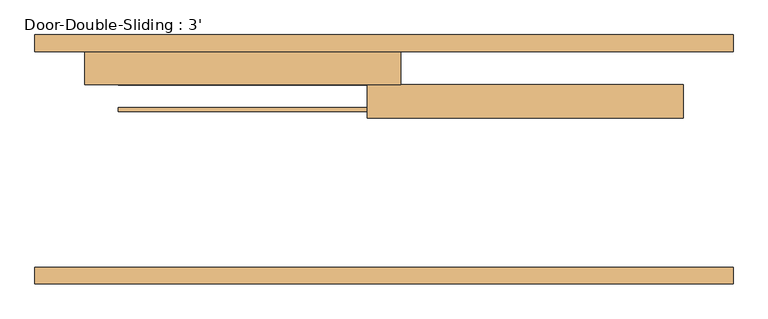
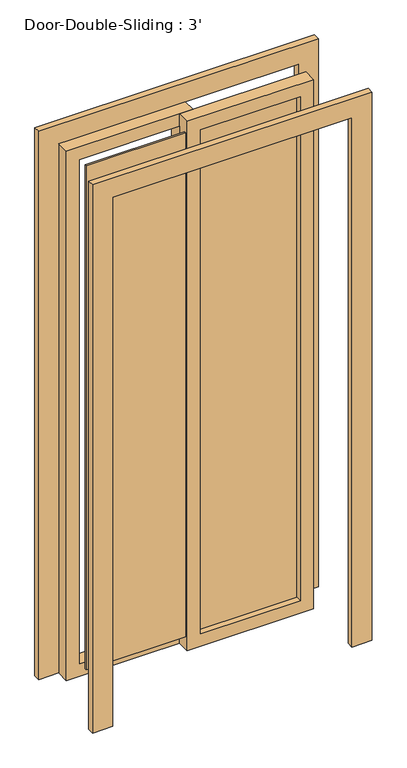
"""IFC4 building model written with IfcOpenShell, lengths in millimetres: door geometry, Door-Double-Sliding : 3'."""

from ifc_helpers import new_model, si_unit, frame, origin, place, context, project, spatial, polyline, outline, extrude, source, transform, mapped, element, save


def door_double_sliding_3_d0d11cef(model_context):
    return source(origin(), model_context, "Body", "SweptSolid", [
        extrude(outline(polyline([(0.0, 533.4), (2209.8, 533.4), (2209.8, -533.4), (0.0, -533.4), (0.0, -457.2), (2133.6, -457.2), (2133.6, 457.2), (0.0, 457.2), (0.0, 533.4)])), frame((0.0, 292.1, 0.0), z_axis=(0.0, 1.0, 0.0), x_axis=(0.0, 0.0, 1.0)), (0.0, 0.0, 1.0), 25.4),
        extrude(outline(polyline([(0.0, -533.4), (0.0, -457.2), (2133.6, -457.2), (2133.6, 457.2), (0.0, 457.2), (0.0, 533.4), (2209.8, 533.4), (2209.8, -533.4), (0.0, -533.4)])), frame((0.0, -63.5, 0.0), z_axis=(0.0, 1.0, 0.0), x_axis=(0.0, 0.0, 1.0)), (0.0, 0.0, 1.0), 25.4),
        extrude(outline(polyline([(2133.6, 25.4), (2133.6, -457.2), (0.0, -457.2), (0.0, 25.4), (2133.6, 25.4)]), holes=[polyline([(2082.8, -25.4), (50.8, -25.4), (50.8, -406.4), (2082.8, -406.4), (2082.8, -25.4)])]), frame((0.0, 241.3, 0.0), z_axis=(0.0, 1.0, 0.0), x_axis=(0.0, 0.0, 1.0)), (0.0, 0.0, 1.0), 50.8),
        extrude(outline(polyline([(2133.6, -25.4), (0.0, -25.4), (0.0, 457.2), (2133.6, 457.2), (2133.6, -25.4)]), holes=[polyline([(2082.8, 25.4), (2082.8, 406.4), (50.8, 406.4), (50.8, 25.4), (2082.8, 25.4)])]), frame((0.0, 190.5, 0.0), z_axis=(0.0, 1.0, 0.0), x_axis=(0.0, 0.0, 1.0)), (0.0, 0.0, 1.0), 50.8),
        extrude(outline(polyline([(-25.4, 200.025), (-406.4, 200.025), (-406.4, 206.375), (-25.4, 206.375), (-25.4, 200.025)])), frame((0.0, 0.0, 50.8), z_axis=(0.0, 0.0, 1.0), x_axis=(1.0, 0.0, 0.0)), (0.0, 0.0, 1.0), 2032.0),
        extrude(outline(polyline([(25.4, 219.075), (406.4, 219.075), (406.4, 212.725), (25.4, 212.725), (25.4, 219.075)])), frame((0.0, 0.0, 50.8), z_axis=(0.0, 0.0, 1.0), x_axis=(1.0, 0.0, 0.0)), (0.0, 0.0, 1.0), 2032.0),
    ])


if __name__ == "__main__":
    model = new_model("IFC4")
    model_context = context("Model", 3, world=origin())
    ifc_project = project(units=[si_unit("LENGTHUNIT", "METRE", prefix="MILLI")], contexts=[model_context])
    site = spatial("IfcSite", under=ifc_project)
    building = spatial("IfcBuilding", under=site)
    placement = place(None, origin())
    door_double_sliding_3_shape = door_double_sliding_3_d0d11cef(model_context)
    element("IfcDoor", 1, ObjectType="Door-Double-Sliding : 3'", at=placement, inside=building, context=model_context, shape_type="MappedRepresentation", body=[
        mapped(door_double_sliding_3_shape, transform((0.0, 0.0, 0.0), x_axis=(1.0, 0.0, 0.0), y_axis=(0.0, 1.0, 0.0), z_axis=(0.0, 0.0, 1.0))),
    ])
    save(model, "model.ifc")

# Revit data of these elements
# Type "Door-Double-Sliding : 3'"
#   Type Mark = "16"
#   Construction Type Id = "opn-d45"
#   Assembly Code = "C1020"
#   Analytic Construction = "Wood frame, double glass door "
#   Thickness = 0' - 2"
#   Thermal Resistance (R) = 1.8150 (h·ft²·°F)/BTU
#   Heat Transfer Coefficient (U) = 0.5510 BTU/(h·ft²·°F)
#   Height = 7' - 0"
#   Rail Width = 0' - 2"
#   Stiles = 0' - 2"
#   Trim Projection Ext = 0' - 1"
#   Trim Projection Int = 0' - 1"
#   Trim Width = 0' - 3"
#   Width = 3' - 0"
#   Define Thermal Properties by = 1
#   Glazing = Glass
#   Panel Material = Wood - Birch - Solid Stained Light Low Gloss
#   Trim Material = Paint - Sienna
#   Visual Light Transmittance = 0
#   Solar Heat Gain Coefficient = 0
#   Function = (empty or 0)
#   Wall Closure = (empty or 0)
# Element 1 (IfcDoor, "Door-Double-Sliding : 3'")
#   Materials on its faces: "Paint - Sienna", "Wood - Birch - Solid Stained Light Low Gloss", "Glass"
# Materials
#   "Glass": class "Glass", colour RGB 0 128 192, transparency 0.75, Description = "Soda Lime Glass", Cost = 0
#   "Wood - Birch - Solid Stained Light Low Gloss": class "Wood", colour RGB 210 159 95, transparency 0, Cost = 0
#   "Paint - Sienna": colour RGB 118 70 51, transparency 0, Cost = 0
